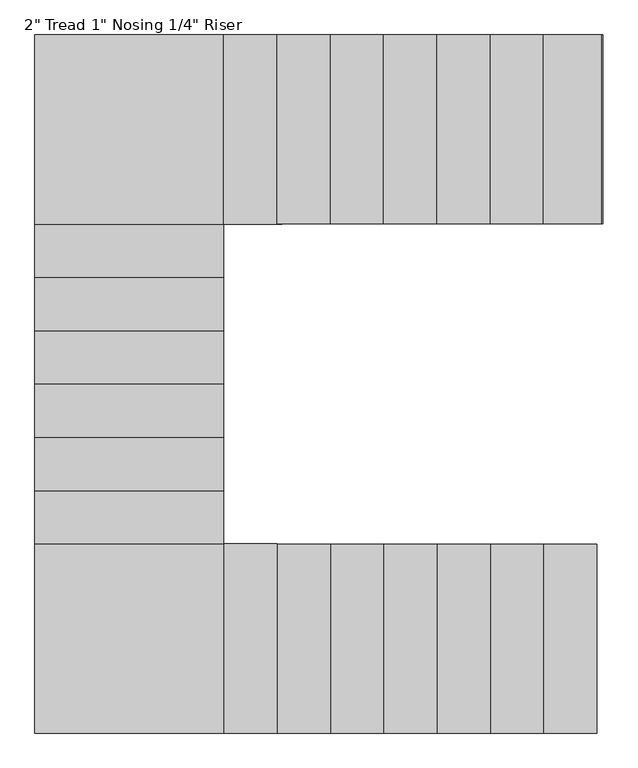
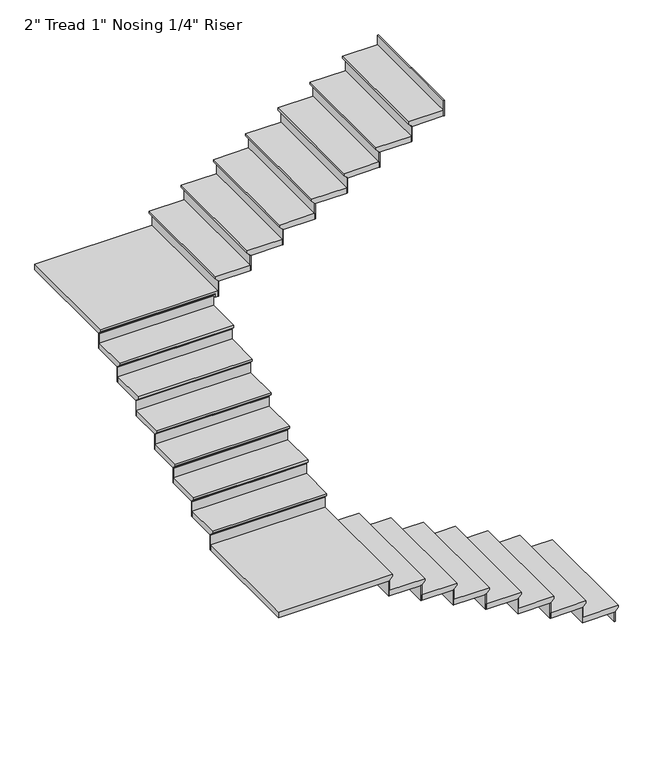
"""IFC4 building model written with IfcOpenShell, lengths in millimetres: stair flight geometry."""

from ifc_helpers import new_model, si_unit, origin, place, context, project, spatial, faceted_brep, source, transform, mapped, element, save


def stair_flight_efd8c866(model_context):
    return source(origin(), model_context, "Body", "Brep", [
        faceted_brep([(-19769.8789184, -127.8399287, 119.4954545), (-19769.8789184, -127.8399287, 138.5454545), (-19769.8789184, -1118.4399287, 138.5454545), (-19769.8789184, -1118.4399287, 119.4954545), (-19795.2789184, -127.8399287, 94.0954545), (-19795.2789184, -1118.4399287, 94.0954545), (-20074.6789184, -127.8399287, 138.5454545), (-20074.6789184, -1118.4399287, 138.5454545), (-19795.2789184, -1118.4399287, 87.7454545), (-20074.6789184, -1118.4399287, 87.7454545), (-20074.6789184, -127.8399287, 87.7454545), (-19795.2789184, -127.8399287, 87.7454545)], [[[0, 1, 2, 3]], [[4, 0, 3, 5]], [[2, 1, 6, 7]], [[8, 9, 10, 11]], [[2, 7, 9, 8, 5, 3]], [[8, 11, 4, 5]], [[6, 1, 0, 4, 11, 10]], [[7, 6, 10, 9]]]),
        faceted_brep([(-19795.2789184, -127.8399287, 87.7454545), (-19795.2789184, -127.8399287, 0.0), (-19801.6289184, -127.8399287, 0.0), (-19801.6289184, -127.8399287, 87.7454545), (-19795.2789184, -1118.4399287, 87.7454545), (-19801.6289184, -1118.4399287, 87.7454545), (-19801.6289184, -1118.4399287, 0.0), (-19795.2789184, -1118.4399287, 0.0)], [[[0, 1, 2, 3]], [[4, 5, 6, 7]], [[1, 0, 4, 7]], [[2, 1, 7, 6]], [[3, 2, 6, 5]], [[0, 3, 5, 4]]]),
        faceted_brep([(-20074.6789184, -127.8399287, 226.2909091), (-20074.6789184, -127.8399287, 87.7454545), (-20081.0289184, -127.8399287, 87.7454545), (-20081.0289184, -127.8399287, 226.2909091), (-20074.6789184, -1118.4399287, 226.2909091), (-20081.0289184, -1118.4399287, 226.2909091), (-20081.0289184, -1118.4399287, 87.7454545), (-20074.6789184, -1118.4399287, 87.7454545)], [[[0, 1, 2, 3]], [[4, 5, 6, 7]], [[1, 0, 4, 7]], [[2, 1, 7, 6]], [[3, 2, 6, 5]], [[0, 3, 5, 4]]]),
        faceted_brep([(-20049.2789184, -1118.4399287, 277.0909091), (-20049.2789184, -127.8399287, 277.0909091), (-20354.0789184, -127.8399287, 277.0909091), (-20354.0789184, -1118.4399287, 277.0909091), (-20074.6789184, -1118.4399287, 226.2909091), (-20354.0789184, -1118.4399287, 226.2909091), (-20354.0789184, -127.8399287, 226.2909091), (-20074.6789184, -127.8399287, 226.2909091), (-20074.6789184, -1118.4399287, 232.6409091), (-20049.2789184, -1118.4399287, 258.0409091), (-20074.6789184, -127.8399287, 232.6409091), (-20049.2789184, -127.8399287, 258.0409091)], [[[0, 1, 2, 3]], [[4, 5, 6, 7]], [[0, 3, 5, 4, 8, 9]], [[4, 7, 10, 8]], [[2, 1, 11, 10, 7, 6]], [[3, 2, 6, 5]], [[11, 1, 0, 9]], [[10, 11, 9, 8]]]),
        faceted_brep([(-20354.0789184, -127.8399287, 364.8363636), (-20354.0789184, -127.8399287, 226.2909091), (-20360.4289184, -127.8399287, 226.2909091), (-20360.4289184, -127.8399287, 364.8363636), (-20354.0789184, -1118.4399287, 364.8363636), (-20360.4289184, -1118.4399287, 364.8363636), (-20360.4289184, -1118.4399287, 226.2909091), (-20354.0789184, -1118.4399287, 226.2909091)], [[[0, 1, 2, 3]], [[4, 5, 6, 7]], [[1, 0, 4, 7]], [[2, 1, 7, 6]], [[3, 2, 6, 5]], [[0, 3, 5, 4]]]),
        faceted_brep([(-20328.6789184, -1118.4399287, 415.6363636), (-20328.6789184, -127.8399287, 415.6363636), (-20633.4789184, -127.8399287, 415.6363636), (-20633.4789184, -1118.4399287, 415.6363636), (-20354.0789184, -1118.4399287, 364.8363636), (-20633.4789184, -1118.4399287, 364.8363636), (-20633.4789184, -127.8399287, 364.8363636), (-20354.0789184, -127.8399287, 364.8363636), (-20354.0789184, -1118.4399287, 371.1863636), (-20328.6789184, -1118.4399287, 396.5863636), (-20354.0789184, -127.8399287, 371.1863636), (-20328.6789184, -127.8399287, 396.5863636)], [[[0, 1, 2, 3]], [[4, 5, 6, 7]], [[0, 3, 5, 4, 8, 9]], [[4, 7, 10, 8]], [[2, 1, 11, 10, 7, 6]], [[3, 2, 6, 5]], [[11, 1, 0, 9]], [[10, 11, 9, 8]]]),
        faceted_brep([(-20633.4789184, -127.8399287, 503.3818182), (-20633.4789184, -127.8399287, 364.8363636), (-20639.8289184, -127.8399287, 364.8363636), (-20639.8289184, -127.8399287, 503.3818182), (-20633.4789184, -1118.4399287, 503.3818182), (-20639.8289184, -1118.4399287, 503.3818182), (-20639.8289184, -1118.4399287, 364.8363636), (-20633.4789184, -1118.4399287, 364.8363636)], [[[0, 1, 2, 3]], [[4, 5, 6, 7]], [[1, 0, 4, 7]], [[2, 1, 7, 6]], [[3, 2, 6, 5]], [[0, 3, 5, 4]]]),
        faceted_brep([(-20608.0789184, -1118.4399287, 554.1818182), (-20608.0789184, -127.8399287, 554.1818182), (-20912.8789184, -127.8399287, 554.1818182), (-20912.8789184, -1118.4399287, 554.1818182), (-20633.4789184, -1118.4399287, 503.3818182), (-20912.8789184, -1118.4399287, 503.3818182), (-20912.8789184, -127.8399287, 503.3818182), (-20633.4789184, -127.8399287, 503.3818182), (-20633.4789184, -1118.4399287, 509.7318182), (-20608.0789184, -1118.4399287, 535.1318182), (-20633.4789184, -127.8399287, 509.7318182), (-20608.0789184, -127.8399287, 535.1318182)], [[[0, 1, 2, 3]], [[4, 5, 6, 7]], [[0, 3, 5, 4, 8, 9]], [[4, 7, 10, 8]], [[2, 1, 11, 10, 7, 6]], [[3, 2, 6, 5]], [[11, 1, 0, 9]], [[10, 11, 9, 8]]]),
        faceted_brep([(-20912.8789184, -127.8399287, 641.9272727), (-20912.8789184, -127.8399287, 503.3818182), (-20919.2289184, -127.8399287, 503.3818182), (-20919.2289184, -127.8399287, 641.9272727), (-20912.8789184, -1118.4399287, 641.9272727), (-20919.2289184, -1118.4399287, 641.9272727), (-20919.2289184, -1118.4399287, 503.3818182), (-20912.8789184, -1118.4399287, 503.3818182)], [[[0, 1, 2, 3]], [[4, 5, 6, 7]], [[1, 0, 4, 7]], [[2, 1, 7, 6]], [[3, 2, 6, 5]], [[0, 3, 5, 4]]]),
        faceted_brep([(-20887.4789184, -1118.4399287, 692.7272727), (-20887.4789184, -127.8399287, 692.7272727), (-21192.2789184, -127.8399287, 692.7272727), (-21192.2789184, -1118.4399287, 692.7272727), (-20912.8789184, -1118.4399287, 641.9272727), (-21192.2789184, -1118.4399287, 641.9272727), (-21192.2789184, -127.8399287, 641.9272727), (-20912.8789184, -127.8399287, 641.9272727), (-20912.8789184, -1118.4399287, 648.2772727), (-20887.4789184, -1118.4399287, 673.6772727), (-20912.8789184, -127.8399287, 648.2772727), (-20887.4789184, -127.8399287, 673.6772727)], [[[0, 1, 2, 3]], [[4, 5, 6, 7]], [[0, 3, 5, 4, 8, 9]], [[4, 7, 10, 8]], [[2, 1, 11, 10, 7, 6]], [[3, 2, 6, 5]], [[11, 1, 0, 9]], [[10, 11, 9, 8]]]),
        faceted_brep([(-21192.2789184, -127.8399287, 780.4727273), (-21192.2789184, -127.8399287, 641.9272727), (-21198.6289184, -127.8399287, 641.9272727), (-21198.6289184, -127.8399287, 780.4727273), (-21192.2789184, -1118.4399287, 780.4727273), (-21198.6289184, -1118.4399287, 780.4727273), (-21198.6289184, -1118.4399287, 641.9272727), (-21192.2789184, -1118.4399287, 641.9272727)], [[[0, 1, 2, 3]], [[4, 5, 6, 7]], [[1, 0, 4, 7]], [[2, 1, 7, 6]], [[3, 2, 6, 5]], [[0, 3, 5, 4]]]),
        faceted_brep([(-21166.8789184, -1118.4399287, 831.2727273), (-21166.8789184, -127.8399287, 831.2727273), (-21471.6789184, -127.8399287, 831.2727273), (-21471.6789184, -1118.4399287, 831.2727273), (-21192.2789184, -1118.4399287, 780.4727273), (-21471.6789184, -1118.4399287, 780.4727273), (-21471.6789184, -127.8399287, 780.4727273), (-21192.2789184, -127.8399287, 780.4727273), (-21192.2789184, -1118.4399287, 786.8227273), (-21166.8789184, -1118.4399287, 812.2227273), (-21192.2789184, -127.8399287, 786.8227273), (-21166.8789184, -127.8399287, 812.2227273)], [[[0, 1, 2, 3]], [[4, 5, 6, 7]], [[0, 3, 5, 4, 8, 9]], [[4, 7, 10, 8]], [[2, 1, 11, 10, 7, 6]], [[3, 2, 6, 5]], [[11, 1, 0, 9]], [[10, 11, 9, 8]]]),
        faceted_brep([(-21471.6789184, -127.8399287, 919.0181818), (-21471.6789184, -127.8399287, 780.4727273), (-21478.0289184, -127.8399287, 780.4727273), (-21478.0289184, -127.8399287, 919.0181818), (-21471.6789184, -1118.4399287, 919.0181818), (-21478.0289184, -1118.4399287, 919.0181818), (-21478.0289184, -1118.4399287, 780.4727273), (-21471.6789184, -1118.4399287, 780.4727273)], [[[0, 1, 2, 3]], [[4, 5, 6, 7]], [[1, 0, 4, 7]], [[2, 1, 7, 6]], [[3, 2, 6, 5]], [[0, 3, 5, 4]]]),
        faceted_brep([(-21446.2789184, -1118.4399287, 969.8181818), (-21446.2789184, -127.8399287, 969.8181818), (-21751.0789184, -127.8399287, 969.8181818), (-21751.0789184, -1118.4399287, 969.8181818), (-21471.6789184, -1118.4399287, 919.0181818), (-21751.0789184, -1118.4399287, 919.0181818), (-21751.0789184, -127.8399287, 919.0181818), (-21471.6789184, -127.8399287, 919.0181818), (-21471.6789184, -1118.4399287, 925.3681818), (-21446.2789184, -1118.4399287, 950.7681818), (-21471.6789184, -127.8399287, 925.3681818), (-21446.2789184, -127.8399287, 950.7681818)], [[[0, 1, 2, 3]], [[4, 5, 6, 7]], [[0, 3, 5, 4, 8, 9]], [[4, 7, 10, 8]], [[2, 1, 11, 10, 7, 6]], [[3, 2, 6, 5]], [[11, 1, 0, 9]], [[10, 11, 9, 8]]]),
        faceted_brep([(-21751.0789184, -127.8399287, 1057.5636364), (-21751.0789184, -127.8399287, 919.0181818), (-21757.4289184, -127.8399287, 919.0181818), (-21757.4289184, -127.8399287, 1057.5636364), (-21751.0789184, -1118.4399287, 1057.5636364), (-21757.4289184, -1118.4399287, 1057.5636364), (-21757.4289184, -1118.4399287, 919.0181818), (-21751.0789184, -1118.4399287, 919.0181818)], [[[0, 1, 2, 3]], [[4, 5, 6, 7]], [[1, 0, 4, 7]], [[2, 1, 7, 6]], [[3, 2, 6, 5]], [[0, 3, 5, 4]]]),
        faceted_brep([(-22716.2789184, -102.4399287, 1108.3636364), (-22716.2789184, -1118.4399287, 1108.3636364), (-21725.6789184, -1118.4399287, 1108.3636364), (-21725.6789184, -102.4399287, 1108.3636364), (-22716.2789184, -1118.4399287, 1057.5636364), (-22716.2789184, -102.4399287, 1057.5636364), (-21725.6789184, -102.4399287, 1057.5636364), (-21725.6789184, -127.8399287, 1057.5636364), (-21751.0789184, -127.8399287, 1057.5636364), (-21751.0789184, -1118.4399287, 1057.5636364), (-21751.0789184, -127.8399287, 1063.9136364), (-21751.0789184, -1118.4399287, 1063.9136364), (-21725.6789184, -1118.4399287, 1089.3136364), (-21725.6789184, -127.8399287, 1089.3136364)], [[[0, 1, 2, 3]], [[4, 5, 6, 7, 8, 9]], [[1, 0, 5, 4]], [[9, 8, 10, 11]], [[3, 2, 12, 13, 7, 6]], [[0, 3, 6, 5]], [[12, 11, 10, 13]], [[2, 1, 4, 9, 11, 12]], [[8, 7, 13, 10]]]),
        faceted_brep([(-21725.6789184, -102.4399287, 1196.1090909), (-21725.6789184, -102.4399287, 1057.5636364), (-21725.6789184, -96.0899287, 1057.5636364), (-21725.6789184, -96.0899287, 1196.1090909), (-22716.2789184, -102.4399287, 1196.1090909), (-22716.2789184, -96.0899287, 1196.1090909), (-22716.2789184, -96.0899287, 1057.5636364), (-22716.2789184, -102.4399287, 1057.5636364)], [[[0, 1, 2, 3]], [[4, 5, 6, 7]], [[1, 0, 4, 7]], [[2, 1, 7, 6]], [[3, 2, 6, 5]], [[0, 3, 5, 4]]]),
        faceted_brep([(-22716.2789184, -127.8399287, 1246.9090909), (-21725.6789184, -127.8399287, 1246.9090909), (-21725.6789184, 176.9600713, 1246.9090909), (-22716.2789184, 176.9600713, 1246.9090909), (-22716.2789184, -102.4399287, 1196.1090909), (-22716.2789184, 176.9600713, 1196.1090909), (-21725.6789184, 176.9600713, 1196.1090909), (-21725.6789184, -102.4399287, 1196.1090909), (-22716.2789184, -102.4399287, 1202.4590909), (-22716.2789184, -127.8399287, 1227.8590909), (-21725.6789184, -102.4399287, 1202.4590909), (-21725.6789184, -127.8399287, 1227.8590909)], [[[0, 1, 2, 3]], [[4, 5, 6, 7]], [[0, 3, 5, 4, 8, 9]], [[4, 7, 10, 8]], [[2, 1, 11, 10, 7, 6]], [[3, 2, 6, 5]], [[11, 1, 0, 9]], [[10, 11, 9, 8]]]),
        faceted_brep([(-21725.6789184, 176.9600713, 1334.6545455), (-21725.6789184, 176.9600713, 1196.1090909), (-21725.6789184, 183.3100713, 1196.1090909), (-21725.6789184, 183.3100713, 1334.6545455), (-22716.2789184, 176.9600713, 1334.6545455), (-22716.2789184, 183.3100713, 1334.6545455), (-22716.2789184, 183.3100713, 1196.1090909), (-22716.2789184, 176.9600713, 1196.1090909)], [[[0, 1, 2, 3]], [[4, 5, 6, 7]], [[1, 0, 4, 7]], [[2, 1, 7, 6]], [[3, 2, 6, 5]], [[0, 3, 5, 4]]]),
        faceted_brep([(-22716.2789184, 151.5600713, 1385.4545455), (-21725.6789184, 151.5600713, 1385.4545455), (-21725.6789184, 456.3600713, 1385.4545455), (-22716.2789184, 456.3600713, 1385.4545455), (-22716.2789184, 176.9600713, 1334.6545455), (-22716.2789184, 456.3600713, 1334.6545455), (-21725.6789184, 456.3600713, 1334.6545455), (-21725.6789184, 176.9600713, 1334.6545455), (-22716.2789184, 176.9600713, 1341.0045455), (-22716.2789184, 151.5600713, 1366.4045455), (-21725.6789184, 176.9600713, 1341.0045455), (-21725.6789184, 151.5600713, 1366.4045455)], [[[0, 1, 2, 3]], [[4, 5, 6, 7]], [[0, 3, 5, 4, 8, 9]], [[4, 7, 10, 8]], [[2, 1, 11, 10, 7, 6]], [[3, 2, 6, 5]], [[11, 1, 0, 9]], [[10, 11, 9, 8]]]),
        faceted_brep([(-21725.6789184, 456.3600713, 1473.2), (-21725.6789184, 456.3600713, 1334.6545455), (-21725.6789184, 462.7100713, 1334.6545455), (-21725.6789184, 462.7100713, 1473.2), (-22716.2789184, 456.3600713, 1473.2), (-22716.2789184, 462.7100713, 1473.2), (-22716.2789184, 462.7100713, 1334.6545455), (-22716.2789184, 456.3600713, 1334.6545455)], [[[0, 1, 2, 3]], [[4, 5, 6, 7]], [[1, 0, 4, 7]], [[2, 1, 7, 6]], [[3, 2, 6, 5]], [[0, 3, 5, 4]]]),
        faceted_brep([(-22716.2789184, 430.9600713, 1524.0), (-21725.6789184, 430.9600713, 1524.0), (-21725.6789184, 735.7600713, 1524.0), (-22716.2789184, 735.7600713, 1524.0), (-22716.2789184, 456.3600713, 1473.2), (-22716.2789184, 735.7600713, 1473.2), (-21725.6789184, 735.7600713, 1473.2), (-21725.6789184, 456.3600713, 1473.2), (-22716.2789184, 456.3600713, 1479.55), (-22716.2789184, 430.9600713, 1504.95), (-21725.6789184, 456.3600713, 1479.55), (-21725.6789184, 430.9600713, 1504.95)], [[[0, 1, 2, 3]], [[4, 5, 6, 7]], [[0, 3, 5, 4, 8, 9]], [[4, 7, 10, 8]], [[2, 1, 11, 10, 7, 6]], [[3, 2, 6, 5]], [[11, 1, 0, 9]], [[10, 11, 9, 8]]]),
        faceted_brep([(-21725.6789184, 735.7600713, 1611.7454545), (-21725.6789184, 735.7600713, 1473.2), (-21725.6789184, 742.1100713, 1473.2), (-21725.6789184, 742.1100713, 1611.7454545), (-22716.2789184, 735.7600713, 1611.7454545), (-22716.2789184, 742.1100713, 1611.7454545), (-22716.2789184, 742.1100713, 1473.2), (-22716.2789184, 735.7600713, 1473.2)], [[[0, 1, 2, 3]], [[4, 5, 6, 7]], [[1, 0, 4, 7]], [[2, 1, 7, 6]], [[3, 2, 6, 5]], [[0, 3, 5, 4]]]),
        faceted_brep([(-22716.2789184, 710.3600713, 1662.5454545), (-21725.6789184, 710.3600713, 1662.5454545), (-21725.6789184, 1015.1600713, 1662.5454545), (-22716.2789184, 1015.1600713, 1662.5454545), (-22716.2789184, 735.7600713, 1611.7454545), (-22716.2789184, 1015.1600713, 1611.7454545), (-21725.6789184, 1015.1600713, 1611.7454545), (-21725.6789184, 735.7600713, 1611.7454545), (-22716.2789184, 735.7600713, 1618.0954545), (-22716.2789184, 710.3600713, 1643.4954545), (-21725.6789184, 735.7600713, 1618.0954545), (-21725.6789184, 710.3600713, 1643.4954545)], [[[0, 1, 2, 3]], [[4, 5, 6, 7]], [[0, 3, 5, 4, 8, 9]], [[4, 7, 10, 8]], [[2, 1, 11, 10, 7, 6]], [[3, 2, 6, 5]], [[11, 1, 0, 9]], [[10, 11, 9, 8]]]),
        faceted_brep([(-21725.6789184, 1015.1600713, 1750.2909091), (-21725.6789184, 1015.1600713, 1611.7454545), (-21725.6789184, 1021.5100713, 1611.7454545), (-21725.6789184, 1021.5100713, 1750.2909091), (-22716.2789184, 1015.1600713, 1750.2909091), (-22716.2789184, 1021.5100713, 1750.2909091), (-22716.2789184, 1021.5100713, 1611.7454545), (-22716.2789184, 1015.1600713, 1611.7454545)], [[[0, 1, 2, 3]], [[4, 5, 6, 7]], [[1, 0, 4, 7]], [[2, 1, 7, 6]], [[3, 2, 6, 5]], [[0, 3, 5, 4]]]),
        faceted_brep([(-22716.2789184, 989.7600713, 1801.0909091), (-21725.6789184, 989.7600713, 1801.0909091), (-21725.6789184, 1294.5600713, 1801.0909091), (-22716.2789184, 1294.5600713, 1801.0909091), (-22716.2789184, 1015.1600713, 1750.2909091), (-22716.2789184, 1294.5600713, 1750.2909091), (-21725.6789184, 1294.5600713, 1750.2909091), (-21725.6789184, 1015.1600713, 1750.2909091), (-22716.2789184, 1015.1600713, 1756.6409091), (-22716.2789184, 989.7600713, 1782.0409091), (-21725.6789184, 1015.1600713, 1756.6409091), (-21725.6789184, 989.7600713, 1782.0409091)], [[[0, 1, 2, 3]], [[4, 5, 6, 7]], [[0, 3, 5, 4, 8, 9]], [[4, 7, 10, 8]], [[2, 1, 11, 10, 7, 6]], [[3, 2, 6, 5]], [[11, 1, 0, 9]], [[10, 11, 9, 8]]]),
        faceted_brep([(-21725.6789184, 1294.5600713, 1888.8363636), (-21725.6789184, 1294.5600713, 1750.2909091), (-21725.6789184, 1300.9100713, 1750.2909091), (-21725.6789184, 1300.9100713, 1888.8363636), (-22716.2789184, 1294.5600713, 1888.8363636), (-22716.2789184, 1300.9100713, 1888.8363636), (-22716.2789184, 1300.9100713, 1750.2909091), (-22716.2789184, 1294.5600713, 1750.2909091)], [[[0, 1, 2, 3]], [[4, 5, 6, 7]], [[1, 0, 4, 7]], [[2, 1, 7, 6]], [[3, 2, 6, 5]], [[0, 3, 5, 4]]]),
        faceted_brep([(-22716.2789184, 1269.1600713, 1939.6363636), (-21725.6789184, 1269.1600713, 1939.6363636), (-21725.6789184, 1573.9600713, 1939.6363636), (-22716.2789184, 1573.9600713, 1939.6363636), (-22716.2789184, 1294.5600713, 1888.8363636), (-22716.2789184, 1573.9600713, 1888.8363636), (-21725.6789184, 1573.9600713, 1888.8363636), (-21725.6789184, 1294.5600713, 1888.8363636), (-22716.2789184, 1294.5600713, 1895.1863636), (-22716.2789184, 1269.1600713, 1920.5863636), (-21725.6789184, 1294.5600713, 1895.1863636), (-21725.6789184, 1269.1600713, 1920.5863636)], [[[0, 1, 2, 3]], [[4, 5, 6, 7]], [[0, 3, 5, 4, 8, 9]], [[4, 7, 10, 8]], [[2, 1, 11, 10, 7, 6]], [[3, 2, 6, 5]], [[11, 1, 0, 9]], [[10, 11, 9, 8]]]),
        faceted_brep([(-21725.6789184, 1573.9600713, 2027.3818182), (-21725.6789184, 1573.9600713, 1888.8363636), (-21725.6789184, 1580.3100713, 1888.8363636), (-21725.6789184, 1580.3100713, 2027.3818182), (-22716.2789184, 1573.9600713, 2027.3818182), (-22716.2789184, 1580.3100713, 2027.3818182), (-22716.2789184, 1580.3100713, 1888.8363636), (-22716.2789184, 1573.9600713, 1888.8363636)], [[[0, 1, 2, 3]], [[4, 5, 6, 7]], [[1, 0, 4, 7]], [[2, 1, 7, 6]], [[3, 2, 6, 5]], [[0, 3, 5, 4]]]),
        faceted_brep([(-21700.2789184, 2539.1600713, 2078.1818182), (-22716.2789184, 2539.1600713, 2078.1818182), (-22716.2789184, 1548.5600713, 2078.1818182), (-21700.2789184, 1548.5600713, 2078.1818182), (-22716.2789184, 2539.1600713, 2027.3818182), (-21700.2789184, 2539.1600713, 2027.3818182), (-21700.2789184, 1548.5600713, 2027.3818182), (-21725.6789184, 1548.5600713, 2027.3818182), (-21725.6789184, 1573.9600713, 2027.3818182), (-22716.2789184, 1573.9600713, 2027.3818182), (-21725.6789184, 1573.9600713, 2033.7318182), (-22716.2789184, 1573.9600713, 2033.7318182), (-22716.2789184, 1548.5600713, 2059.1318182), (-21725.6789184, 1548.5600713, 2059.1318182)], [[[0, 1, 2, 3]], [[4, 5, 6, 7, 8, 9]], [[1, 0, 5, 4]], [[9, 8, 10, 11]], [[3, 2, 12, 13, 7, 6]], [[0, 3, 6, 5]], [[12, 11, 10, 13]], [[2, 1, 4, 9, 11, 12]], [[8, 7, 13, 10]]]),
        faceted_brep([(-21700.2789184, 1548.5600713, 2165.9272727), (-21700.2789184, 1548.5600713, 2027.3818182), (-21693.9289184, 1548.5600713, 2027.3818182), (-21693.9289184, 1548.5600713, 2165.9272727), (-21700.2789184, 2539.1600713, 2165.9272727), (-21693.9289184, 2539.1600713, 2165.9272727), (-21693.9289184, 2539.1600713, 2027.3818182), (-21700.2789184, 2539.1600713, 2027.3818182)], [[[0, 1, 2, 3]], [[4, 5, 6, 7]], [[1, 0, 4, 7]], [[2, 1, 7, 6]], [[3, 2, 6, 5]], [[0, 3, 5, 4]]]),
        faceted_brep([(-21725.6789184, 2539.1600713, 2216.7272727), (-21725.6789184, 1548.5600713, 2216.7272727), (-21420.8789184, 1548.5600713, 2216.7272727), (-21420.8789184, 2539.1600713, 2216.7272727), (-21700.2789184, 2539.1600713, 2165.9272727), (-21420.8789184, 2539.1600713, 2165.9272727), (-21420.8789184, 1548.5600713, 2165.9272727), (-21700.2789184, 1548.5600713, 2165.9272727), (-21700.2789184, 2539.1600713, 2172.2772727), (-21725.6789184, 2539.1600713, 2197.6772727), (-21700.2789184, 1548.5600713, 2172.2772727), (-21725.6789184, 1548.5600713, 2197.6772727)], [[[0, 1, 2, 3]], [[4, 5, 6, 7]], [[0, 3, 5, 4, 8, 9]], [[4, 7, 10, 8]], [[2, 1, 11, 10, 7, 6]], [[3, 2, 6, 5]], [[11, 1, 0, 9]], [[10, 11, 9, 8]]]),
        faceted_brep([(-21420.8789184, 1548.5600713, 2304.4727273), (-21420.8789184, 1548.5600713, 2165.9272727), (-21414.5289184, 1548.5600713, 2165.9272727), (-21414.5289184, 1548.5600713, 2304.4727273), (-21420.8789184, 2539.1600713, 2304.4727273), (-21414.5289184, 2539.1600713, 2304.4727273), (-21414.5289184, 2539.1600713, 2165.9272727), (-21420.8789184, 2539.1600713, 2165.9272727)], [[[0, 1, 2, 3]], [[4, 5, 6, 7]], [[1, 0, 4, 7]], [[2, 1, 7, 6]], [[3, 2, 6, 5]], [[0, 3, 5, 4]]]),
        faceted_brep([(-21446.2789184, 2539.1600713, 2355.2727273), (-21446.2789184, 1548.5600713, 2355.2727273), (-21141.4789184, 1548.5600713, 2355.2727273), (-21141.4789184, 2539.1600713, 2355.2727273), (-21420.8789184, 2539.1600713, 2304.4727273), (-21141.4789184, 2539.1600713, 2304.4727273), (-21141.4789184, 1548.5600713, 2304.4727273), (-21420.8789184, 1548.5600713, 2304.4727273), (-21420.8789184, 2539.1600713, 2310.8227273), (-21446.2789184, 2539.1600713, 2336.2227273), (-21420.8789184, 1548.5600713, 2310.8227273), (-21446.2789184, 1548.5600713, 2336.2227273)], [[[0, 1, 2, 3]], [[4, 5, 6, 7]], [[0, 3, 5, 4, 8, 9]], [[4, 7, 10, 8]], [[2, 1, 11, 10, 7, 6]], [[3, 2, 6, 5]], [[11, 1, 0, 9]], [[10, 11, 9, 8]]]),
        faceted_brep([(-21141.4789184, 1548.5600713, 2443.0181818), (-21141.4789184, 1548.5600713, 2304.4727273), (-21135.1289184, 1548.5600713, 2304.4727273), (-21135.1289184, 1548.5600713, 2443.0181818), (-21141.4789184, 2539.1600713, 2443.0181818), (-21135.1289184, 2539.1600713, 2443.0181818), (-21135.1289184, 2539.1600713, 2304.4727273), (-21141.4789184, 2539.1600713, 2304.4727273)], [[[0, 1, 2, 3]], [[4, 5, 6, 7]], [[1, 0, 4, 7]], [[2, 1, 7, 6]], [[3, 2, 6, 5]], [[0, 3, 5, 4]]]),
        faceted_brep([(-21166.8789184, 2539.1600713, 2493.8181818), (-21166.8789184, 1548.5600713, 2493.8181818), (-20862.0789184, 1548.5600713, 2493.8181818), (-20862.0789184, 2539.1600713, 2493.8181818), (-21141.4789184, 2539.1600713, 2443.0181818), (-20862.0789184, 2539.1600713, 2443.0181818), (-20862.0789184, 1548.5600713, 2443.0181818), (-21141.4789184, 1548.5600713, 2443.0181818), (-21141.4789184, 2539.1600713, 2449.3681818), (-21166.8789184, 2539.1600713, 2474.7681818), (-21141.4789184, 1548.5600713, 2449.3681818), (-21166.8789184, 1548.5600713, 2474.7681818)], [[[0, 1, 2, 3]], [[4, 5, 6, 7]], [[0, 3, 5, 4, 8, 9]], [[4, 7, 10, 8]], [[2, 1, 11, 10, 7, 6]], [[3, 2, 6, 5]], [[11, 1, 0, 9]], [[10, 11, 9, 8]]]),
        faceted_brep([(-20862.0789184, 1548.5600713, 2581.5636364), (-20862.0789184, 1548.5600713, 2443.0181818), (-20855.7289184, 1548.5600713, 2443.0181818), (-20855.7289184, 1548.5600713, 2581.5636364), (-20862.0789184, 2539.1600713, 2581.5636364), (-20855.7289184, 2539.1600713, 2581.5636364), (-20855.7289184, 2539.1600713, 2443.0181818), (-20862.0789184, 2539.1600713, 2443.0181818)], [[[0, 1, 2, 3]], [[4, 5, 6, 7]], [[1, 0, 4, 7]], [[2, 1, 7, 6]], [[3, 2, 6, 5]], [[0, 3, 5, 4]]]),
        faceted_brep([(-20887.4789184, 2539.1600713, 2632.3636364), (-20887.4789184, 1548.5600713, 2632.3636364), (-20582.6789184, 1548.5600713, 2632.3636364), (-20582.6789184, 2539.1600713, 2632.3636364), (-20862.0789184, 2539.1600713, 2581.5636364), (-20582.6789184, 2539.1600713, 2581.5636364), (-20582.6789184, 1548.5600713, 2581.5636364), (-20862.0789184, 1548.5600713, 2581.5636364), (-20862.0789184, 2539.1600713, 2587.9136364), (-20887.4789184, 2539.1600713, 2613.3136364), (-20862.0789184, 1548.5600713, 2587.9136364), (-20887.4789184, 1548.5600713, 2613.3136364)], [[[0, 1, 2, 3]], [[4, 5, 6, 7]], [[0, 3, 5, 4, 8, 9]], [[4, 7, 10, 8]], [[2, 1, 11, 10, 7, 6]], [[3, 2, 6, 5]], [[11, 1, 0, 9]], [[10, 11, 9, 8]]]),
        faceted_brep([(-20582.6789184, 1548.5600713, 2720.1090909), (-20582.6789184, 1548.5600713, 2581.5636364), (-20576.3289184, 1548.5600713, 2581.5636364), (-20576.3289184, 1548.5600713, 2720.1090909), (-20582.6789184, 2539.1600713, 2720.1090909), (-20576.3289184, 2539.1600713, 2720.1090909), (-20576.3289184, 2539.1600713, 2581.5636364), (-20582.6789184, 2539.1600713, 2581.5636364)], [[[0, 1, 2, 3]], [[4, 5, 6, 7]], [[1, 0, 4, 7]], [[2, 1, 7, 6]], [[3, 2, 6, 5]], [[0, 3, 5, 4]]]),
        faceted_brep([(-20608.0789184, 2539.1600713, 2770.9090909), (-20608.0789184, 1548.5600713, 2770.9090909), (-20303.2789184, 1548.5600713, 2770.9090909), (-20303.2789184, 2539.1600713, 2770.9090909), (-20582.6789184, 2539.1600713, 2720.1090909), (-20303.2789184, 2539.1600713, 2720.1090909), (-20303.2789184, 1548.5600713, 2720.1090909), (-20582.6789184, 1548.5600713, 2720.1090909), (-20582.6789184, 2539.1600713, 2726.4590909), (-20608.0789184, 2539.1600713, 2751.8590909), (-20582.6789184, 1548.5600713, 2726.4590909), (-20608.0789184, 1548.5600713, 2751.8590909)], [[[0, 1, 2, 3]], [[4, 5, 6, 7]], [[0, 3, 5, 4, 8, 9]], [[4, 7, 10, 8]], [[2, 1, 11, 10, 7, 6]], [[3, 2, 6, 5]], [[11, 1, 0, 9]], [[10, 11, 9, 8]]]),
        faceted_brep([(-20303.2789184, 1548.5600713, 2858.6545455), (-20303.2789184, 1548.5600713, 2720.1090909), (-20296.9289184, 1548.5600713, 2720.1090909), (-20296.9289184, 1548.5600713, 2858.6545455), (-20303.2789184, 2539.1600713, 2858.6545455), (-20296.9289184, 2539.1600713, 2858.6545455), (-20296.9289184, 2539.1600713, 2720.1090909), (-20303.2789184, 2539.1600713, 2720.1090909)], [[[0, 1, 2, 3]], [[4, 5, 6, 7]], [[1, 0, 4, 7]], [[2, 1, 7, 6]], [[3, 2, 6, 5]], [[0, 3, 5, 4]]]),
        faceted_brep([(-20328.6789184, 2539.1600713, 2909.4545455), (-20328.6789184, 1548.5600713, 2909.4545455), (-20023.8789184, 1548.5600713, 2909.4545455), (-20023.8789184, 2539.1600713, 2909.4545455), (-20303.2789184, 2539.1600713, 2858.6545455), (-20023.8789184, 2539.1600713, 2858.6545455), (-20023.8789184, 1548.5600713, 2858.6545455), (-20303.2789184, 1548.5600713, 2858.6545455), (-20303.2789184, 2539.1600713, 2865.0045455), (-20328.6789184, 2539.1600713, 2890.4045455), (-20303.2789184, 1548.5600713, 2865.0045455), (-20328.6789184, 1548.5600713, 2890.4045455)], [[[0, 1, 2, 3]], [[4, 5, 6, 7]], [[0, 3, 5, 4, 8, 9]], [[4, 7, 10, 8]], [[2, 1, 11, 10, 7, 6]], [[3, 2, 6, 5]], [[11, 1, 0, 9]], [[10, 11, 9, 8]]]),
        faceted_brep([(-20023.8789184, 1548.5600713, 2997.2), (-20023.8789184, 1548.5600713, 2858.6545455), (-20017.5289184, 1548.5600713, 2858.6545455), (-20017.5289184, 1548.5600713, 2997.2), (-20023.8789184, 2539.1600713, 2997.2), (-20017.5289184, 2539.1600713, 2997.2), (-20017.5289184, 2539.1600713, 2858.6545455), (-20023.8789184, 2539.1600713, 2858.6545455)], [[[0, 1, 2, 3]], [[4, 5, 6, 7]], [[1, 0, 4, 7]], [[2, 1, 7, 6]], [[3, 2, 6, 5]], [[0, 3, 5, 4]]]),
        faceted_brep([(-19744.4789184, 1548.5600713, 3135.7454545), (-19744.4789184, 1548.5600713, 2997.2), (-19738.1289184, 1548.5600713, 2997.2), (-19738.1289184, 1548.5600713, 3135.7454545), (-19744.4789184, 2539.1600713, 3135.7454545), (-19738.1289184, 2539.1600713, 3135.7454545), (-19738.1289184, 2539.1600713, 2997.2), (-19744.4789184, 2539.1600713, 2997.2)], [[[0, 1, 2, 3]], [[4, 5, 6, 7]], [[1, 0, 4, 7]], [[2, 1, 7, 6]], [[3, 2, 6, 5]], [[0, 3, 5, 4]]]),
        faceted_brep([(-20049.2789184, 2539.1600713, 3048.0), (-20049.2789184, 1548.5600713, 3048.0), (-19744.4789184, 1548.5600713, 3048.0), (-19744.4789184, 2539.1600713, 3048.0), (-20023.8789184, 2539.1600713, 2997.2), (-19744.4789184, 2539.1600713, 2997.2), (-19744.4789184, 1548.5600713, 2997.2), (-20023.8789184, 1548.5600713, 2997.2), (-20023.8789184, 2539.1600713, 3003.55), (-20049.2789184, 2539.1600713, 3028.95), (-20023.8789184, 1548.5600713, 3003.55), (-20049.2789184, 1548.5600713, 3028.95)], [[[0, 1, 2, 3]], [[4, 5, 6, 7]], [[0, 3, 5, 4, 8, 9]], [[4, 7, 10, 8]], [[2, 1, 11, 10, 7, 6]], [[3, 2, 6, 5]], [[11, 1, 0, 9]], [[10, 11, 9, 8]]]),
    ])


if __name__ == "__main__":
    model = new_model("IFC4")
    model_context = context("Model", 3, world=origin())
    ifc_project = project(units=[si_unit("LENGTHUNIT", "METRE", prefix="MILLI")], contexts=[model_context])
    site = spatial("IfcSite", under=ifc_project)
    building = spatial("IfcBuilding", under=site)
    placement = place(None, origin())
    stair_flight_shape = stair_flight_efd8c866(model_context)
    element("IfcStairFlight", 1, ObjectType="2\" Tread 1\" Nosing 1/4\" Riser", at=placement, inside=building, context=model_context, shape_type="MappedRepresentation", body=[
        mapped(stair_flight_shape, transform((0.0, 0.0, 0.0), x_axis=(1.0, 0.0, 0.0), y_axis=(0.0, 1.0, 0.0), z_axis=(0.0, 0.0, 1.0))),
    ])
    save(model, "model.ifc")
